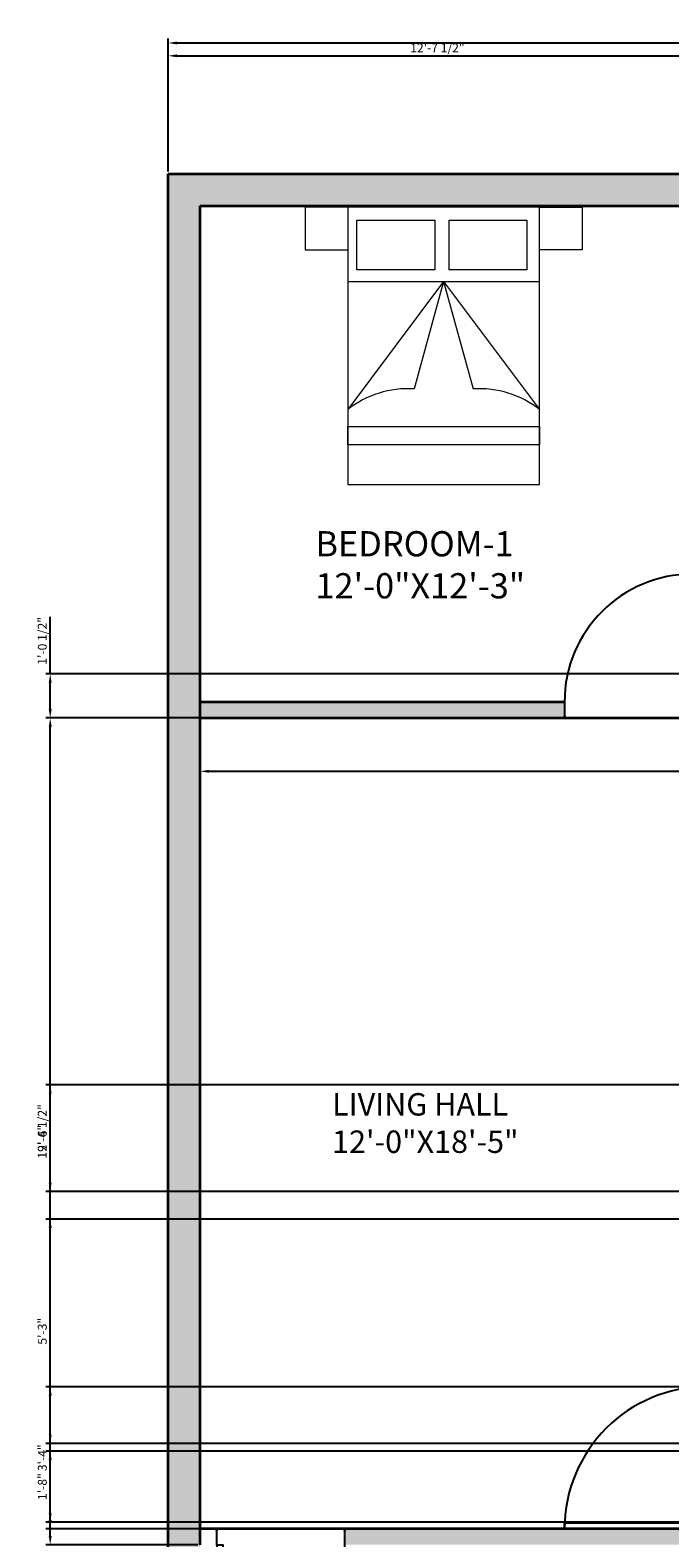
# Model space of a CAD drawing. Units: inches. Extents: x 2063 to 2524, y 2436 to 3097.
# Tile 2 of 4: x 2063 to 2243, y 2673 to 3097. Entities that reach past the tile are written whole.
import ezdxf

# ---------------------------------------------------------------- set-up
doc = ezdxf.new("R2010")
doc.units = ezdxf.units.IN
for name, color, linetype, lineweight in [('A-ANNO-DIMS', 2, 'Continuous', 18), ('A-AREA-IDEN', 7, 'Continuous', 18), ('A-DOOR', 4, 'Continuous', 25), ('A-FURN', 8, 'Continuous', 18), ('A-WALL', 7, 'Continuous', 35)]:
    doc.layers.add(name, color=color, linetype=linetype, lineweight=lineweight)
doc.layers.add('A-WALL-PATT', color=251, linetype='Continuous', lineweight=13, true_color=0x636466)
doc.styles.get("Standard").update_dxf_attribs({"font": 'arial.ttf'})
doc.dimstyles.new('ISO-25', dxfattribs={"dimtxt": 2.5, "dimasz": 2.5, "dimexe": 1.25, "dimexo": 0.625, "dimtad": 1, "dimlunit": 3, "dimtxsty": 'Standard', "dimcen": 2.5, "dimadec": 0, "dimazin": 0, "dimtfac": 1, "dimtmove": 0, "dimatfit": 3, "dimfxl": 1, "dimarcsym": 0})

# ---------------------------------------------------------------- blocks, each defined once
blk = doc.blocks.new('*U3')
for p, q in [((0, 0), (0, -4)), ((-36, 0), (-36, -4))]:
    blk.add_line(p, q)
blk.add_lwpolyline([(0, 0), (0, 36), (-1.75, 36), (-1.75, 0)], close=True)
blk.add_arc((0, 0), 36, 90, 180)
blk = doc.blocks.new('*U5')
for p, q in [((0, 0), (0, -4)), ((40, 0), (40, -4))]:
    blk.add_line(p, q)
blk.add_lwpolyline([(0, 0), (0, 40), (1.75, 40), (1.75, 0)], close=True)
blk.add_arc((0, 0), 40, 0, 90)
blk = doc.blocks.new('*U7')
for p, q in [((0, 0), (0, 4)), ((36, 0), (36, 4))]:
    blk.add_line(p, q)
blk.add_lwpolyline([(0, 0), (0, -36), (1.75, -36), (1.75, 0)], close=True)
blk.add_arc((0, 0), 36, 270, 0)
blk = doc.blocks.new('*D11')
at = {"layer": 'A-ANNO-DIMS', "color": 0, "lineweight": -2, "transparency": 16777216}
for p, q in [((2110.76, 2902.49), (2110.76, 2886.87)), ((2411.76, 2902.49), (2411.76, 2886.87)), ((2113.26, 2888.12), (2409.26, 2888.12))]:
    blk.add_line(p, q, dxfattribs=at)
at = {"layer": 'A-ANNO-DIMS', "color": 0, "transparency": 16777216}
for points in [[(2113.26, 2888.53), (2113.26, 2887.7), (2110.76, 2888.12)], [(2409.26, 2888.53), (2409.26, 2887.7), (2411.76, 2888.12)]]:
    blk.add_solid(points, dxfattribs=at)
at = {"layer": 'Defpoints', "color": 0, "transparency": 16777216}
for p in [(2110.76, 2903.12), (2411.76, 2903.12), (2411.76, 2888.12)]:
    blk.add_point(p, dxfattribs=at)
at = {"layer": 'A-ANNO-DIMS', "color": 0, "transparency": 16777216, "insert": (2261.26, 2890.02), "char_height": 2.5, "attachment_point": 5}
blk.add_mtext('25\'-1"', dxfattribs=at)
blk = doc.blocks.new('*D14')
at = {"layer": 'A-ANNO-DIMS', "color": 0, "lineweight": -2, "transparency": 16777216}
for p, q in [((2101.76, 3056.74), (2101.76, 3094.17)), ((2104.26, 3092.92), (2459.26, 3092.92)), ((2461.76, 3056.74), (2461.76, 3094.17))]:
    blk.add_line(p, q, dxfattribs=at)
at = {"layer": 'A-ANNO-DIMS', "color": 0, "transparency": 16777216}
for points in [[(2104.26, 3093.34), (2104.26, 3092.5), (2101.76, 3092.92)], [(2459.26, 3093.34), (2459.26, 3092.5), (2461.76, 3092.92)]]:
    blk.add_solid(points, dxfattribs=at)
at = {"layer": 'Defpoints', "color": 0, "transparency": 16777216}
for p in [(2461.76, 3092.92), (2101.76, 3056.12), (2461.76, 3056.12)]:
    blk.add_point(p, dxfattribs=at)
at = {"layer": 'A-ANNO-DIMS', "color": 0, "transparency": 16777216, "insert": (2281.76, 3094.82), "char_height": 2.5, "attachment_point": 5}
blk.add_mtext("30'", dxfattribs=at)
blk = doc.blocks.new('BED-DOUBLE-WITH-NIGHTSTANDS')
for p, q in [((12, 78), (0, 78)), ((0, 78), (0, 66)), ((66, 78), (78, 78)), ((78, 78), (78, 66)), ((36.48, 74.39), (36.48, 60.42)), ((40.48, 74.39), (40.48, 60.42)), ((0, 66), (12, 66)), ((77, 66), (66, 66)), ((78, 66), (77, 66)), ((12, 57.08), (66, 57.08)), ((39, 57.08), (12, 21.08)), ((39, 57.08), (30.7, 26.92)), ((39, 57.08), (66, 21.08)), ((39, 57.08), (47.3, 26.92))]:
    blk.add_line(p, q)
for points in [[(12, 0), (66, 0), (66, 78), (12, 78)], [(12, 16.31), (66, 16.31), (66, 11.16), (12, 11.16)]]:
    blk.add_lwpolyline(points, close=True)
for points in [[(36.48, 60.42), (14.53, 60.42), (14.53, 74.39), (36.48, 74.39)], [(40.48, 74.39), (62.43, 74.39), (62.43, 60.42), (40.48, 60.42)]]:
    blk.add_lwpolyline(points)
for centre, start, end in [((29, -0.5), 86.4578, 128.2353), ((49, -0.5), 51.7647, 93.5422)]:
    blk.add_arc(centre, 27.47, start, end)
blk = doc.blocks.new('*D31')
at = {"layer": 'A-ANNO-DIMS', "color": 0, "lineweight": -2, "transparency": 16777216}
for p, q in [((2110.14, 2903.12), (2067.31, 2903.12)), ((2068.56, 2673.12), (2068.56, 2900.62)), ((2110.14, 2670.62), (2067.31, 2670.62))]:
    blk.add_line(p, q, dxfattribs=at)
at = {"layer": 'A-ANNO-DIMS', "color": 0, "transparency": 16777216}
for points in [[(2068.15, 2900.62), (2068.98, 2900.62), (2068.56, 2903.12)], [(2068.15, 2673.12), (2068.98, 2673.12), (2068.56, 2670.62)]]:
    blk.add_solid(points, dxfattribs=at)
at = {"layer": 'Defpoints', "color": 0, "transparency": 16777216}
for p in [(2068.56, 2903.12), (2110.76, 2903.12), (2110.76, 2670.62)]:
    blk.add_point(p, dxfattribs=at)
at = {"layer": 'A-ANNO-DIMS', "color": 0, "transparency": 16777216, "insert": (2066.65, 2786.87), "char_height": 2.5, "attachment_point": 5, "rotation": 90}
blk.add_mtext('19\'-4 1/2"', dxfattribs=at)
blk = doc.blocks.new('*D32')
at = {"layer": 'A-ANNO-DIMS', "color": 0, "lineweight": -2, "transparency": 16777216}
for p, q in [((2101.76, 3056.74), (2101.76, 3090.57)), ((2253.26, 3047.74), (2253.26, 3090.57)), ((2104.26, 3089.32), (2250.76, 3089.32))]:
    blk.add_line(p, q, dxfattribs=at)
at = {"layer": 'A-ANNO-DIMS', "color": 0, "transparency": 16777216}
for points in [[(2104.26, 3089.73), (2104.26, 3088.9), (2101.76, 3089.32)], [(2250.76, 3089.73), (2250.76, 3088.9), (2253.26, 3089.32)]]:
    blk.add_solid(points, dxfattribs=at)
at = {"layer": 'Defpoints', "color": 0, "transparency": 16777216}
for p in [(2253.26, 3089.32), (2101.76, 3056.12), (2253.26, 3047.12)]:
    blk.add_point(p, dxfattribs=at)
at = {"layer": 'A-ANNO-DIMS', "color": 0, "transparency": 16777216, "insert": (2177.51, 3091.24), "char_height": 2.5, "attachment_point": 5}
blk.add_mtext('12\'-7 1/2"', dxfattribs=at)
blk = doc.blocks.new('*D35')
at = {"layer": 'A-ANNO-DIMS', "color": 0, "lineweight": -2, "transparency": 16777216}
for p, q in [((2068.56, 2915.57), (2068.56, 2931.55)), ((2257.14, 2915.57), (2067.31, 2915.57)), ((2068.56, 2905.62), (2068.56, 2913.07)), ((2257.14, 2903.12), (2067.31, 2903.12))]:
    blk.add_line(p, q, dxfattribs=at)
at = {"layer": 'A-ANNO-DIMS', "color": 0, "transparency": 16777216}
for points in [[(2068.15, 2913.07), (2068.98, 2913.07), (2068.56, 2915.57)], [(2068.15, 2905.62), (2068.98, 2905.62), (2068.56, 2903.12)]]:
    blk.add_solid(points, dxfattribs=at)
at = {"layer": 'Defpoints', "color": 0, "transparency": 16777216}
for p in [(2068.56, 2915.57), (2257.76, 2915.57), (2257.76, 2903.12)]:
    blk.add_point(p, dxfattribs=at)
at = {"layer": 'A-ANNO-DIMS', "color": 0, "transparency": 16777216, "insert": (2066.65, 2924.81), "char_height": 2.5, "attachment_point": 5, "rotation": 90}
blk.add_mtext('1\'-0 1/2"', dxfattribs=at)
blk = doc.blocks.new('*D41')
at = {"layer": 'A-ANNO-DIMS', "color": 0, "lineweight": -2, "transparency": 16777216}
for p, q in [((2305.15, 2799.95), (2067.31, 2799.95)), ((2068.56, 2772.45), (2068.56, 2797.45)), ((2305.14, 2769.95), (2067.31, 2769.95))]:
    blk.add_line(p, q, dxfattribs=at)
at = {"layer": 'A-ANNO-DIMS', "color": 0, "transparency": 16777216}
for points in [[(2068.15, 2797.45), (2068.98, 2797.45), (2068.56, 2799.95)], [(2068.15, 2772.45), (2068.98, 2772.45), (2068.56, 2769.95)]]:
    blk.add_solid(points, dxfattribs=at)
at = {"layer": 'Defpoints', "color": 0, "transparency": 16777216}
for p in [(2068.56, 2799.95), (2305.78, 2799.95), (2305.76, 2769.95)]:
    blk.add_point(p, dxfattribs=at)
at = {"layer": 'A-ANNO-DIMS', "color": 0, "transparency": 16777216, "insert": (2066.66, 2784.95), "char_height": 2.5, "attachment_point": 5, "rotation": 90}
blk.add_mtext('2\'-6"', dxfattribs=at)
blk = doc.blocks.new('*D42')
at = {"layer": 'A-ANNO-DIMS', "color": 0, "lineweight": -2, "transparency": 16777216}
for p, q in [((2426.27, 2762.21), (2067.31, 2762.21)), ((2068.56, 2701.62), (2068.56, 2759.71)), ((2426.27, 2699.12), (2067.31, 2699.12))]:
    blk.add_line(p, q, dxfattribs=at)
at = {"layer": 'A-ANNO-DIMS', "color": 0, "transparency": 16777216}
for points in [[(2068.15, 2759.71), (2068.98, 2759.71), (2068.56, 2762.21)], [(2068.15, 2701.62), (2068.98, 2701.62), (2068.56, 2699.12)]]:
    blk.add_solid(points, dxfattribs=at)
at = {"layer": 'Defpoints', "color": 0, "transparency": 16777216}
for p in [(2068.56, 2762.21), (2426.9, 2762.21), (2426.9, 2699.12)]:
    blk.add_point(p, dxfattribs=at)
at = {"layer": 'A-ANNO-DIMS', "color": 0, "transparency": 16777216, "insert": (2066.66, 2730.67), "char_height": 2.5, "attachment_point": 5, "rotation": 90}
blk.add_mtext('5\'-3"', dxfattribs=at)
blk = doc.blocks.new('*D45')
at = {"layer": 'A-ANNO-DIMS', "color": 0, "lineweight": -2, "transparency": 16777216}
for p, q in [((2252.63, 2715.09), (2067.31, 2715.09)), ((2068.56, 2677.62), (2068.56, 2712.59)), ((2252.64, 2675.12), (2067.31, 2675.12))]:
    blk.add_line(p, q, dxfattribs=at)
at = {"layer": 'A-ANNO-DIMS', "color": 0, "transparency": 16777216}
for points in [[(2068.15, 2712.59), (2068.98, 2712.59), (2068.56, 2715.09)], [(2068.15, 2677.62), (2068.98, 2677.62), (2068.56, 2675.12)]]:
    blk.add_solid(points, dxfattribs=at)
at = {"layer": 'Defpoints', "color": 0, "transparency": 16777216}
for p in [(2068.56, 2715.09), (2253.26, 2715.09), (2253.26, 2675.12)]:
    blk.add_point(p, dxfattribs=at)
at = {"layer": 'A-ANNO-DIMS', "color": 0, "transparency": 16777216, "insert": (2066.66, 2695.1), "char_height": 2.5, "attachment_point": 5, "rotation": 90}
blk.add_mtext('3\'-4"', dxfattribs=at)
blk = doc.blocks.new('*D50')
at = {"layer": 'A-ANNO-DIMS', "color": 0, "lineweight": -2, "transparency": 16777216}
for p, q in [((2334.17, 2696.99), (2067.31, 2696.99)), ((2068.56, 2679.49), (2068.56, 2694.49)), ((2334.17, 2676.99), (2067.31, 2676.99))]:
    blk.add_line(p, q, dxfattribs=at)
at = {"layer": 'A-ANNO-DIMS', "color": 0, "transparency": 16777216}
for points in [[(2068.15, 2694.49), (2068.98, 2694.49), (2068.56, 2696.99)], [(2068.15, 2679.49), (2068.98, 2679.49), (2068.56, 2676.99)]]:
    blk.add_solid(points, dxfattribs=at)
at = {"layer": 'Defpoints', "color": 0, "transparency": 16777216}
for p in [(2068.56, 2696.99), (2334.8, 2696.99), (2334.8, 2676.99)]:
    blk.add_point(p, dxfattribs=at)
at = {"layer": 'A-ANNO-DIMS', "color": 0, "transparency": 16777216, "insert": (2066.66, 2686.99), "char_height": 2.5, "attachment_point": 5, "rotation": 90}
blk.add_mtext('1\'-8"', dxfattribs=at)

msp = doc.modelspace()

# ---------------------------------------------------------------- hatches: boundary and pattern name
at = {"layer": 'A-WALL-PATT'}
h = msp.add_hatch(color=256, dxfattribs=at)
h.dxf.hatch_style = 1
h.paths.add_polyline_path([(2110.763, 2670.618), (2110.763, 2676.643), (2110.763, 3047.118), (2452.763, 3047.118), (2452.763, 2501.118), (2200.478, 2501.118), (2200.478, 2492.118), (2461.763, 2492.118), (2461.763, 3056.118), (2101.763, 3056.118), (2101.763, 2492.118), (2149.478, 2492.118), (2149.478, 2496.618), (2149.478, 2501.118), (2110.763, 2501.118)])
h.paths.add_polyline_path([(2257.763, 2675.118), (2257.255, 2675.091), (2253.255, 2675.091), (2213.255, 2675.091), (2151.474, 2675.107), (2151.474, 2674.543), (2151.474, 2670.618), (2253.263, 2670.618), (2253.263, 2501.118), (2257.763, 2501.118)], flags=17)
h.paths.add_polyline_path([(2310.263, 3006.972), (2305.763, 3006.972), (2305.763, 2920.067), (2301.763, 2920.067), (2301.759, 2920.067), (2301.759, 2920.063), (2301.759, 2916.063), (2301.759, 2915.567), (2305.763, 2915.567), (2305.763, 2903.118), (2314.3, 2903.118), (2314.3, 2903.618), (2314.3, 2907.618), (2310.263, 2907.618)], flags=17)
h.paths.add_polyline_path([(2257.763, 3006.972), (2253.263, 3006.972), (2253.263, 2907.618), (2249.263, 2907.618), (2249.258, 2907.618), (2249.258, 2907.597), (2249.258, 2903.597), (2249.258, 2903.118), (2257.763, 2903.118), (2257.763, 2915.567), (2271.759, 2915.567), (2271.759, 2916.063), (2271.759, 2920.067), (2257.763, 2920.067)], flags=17)
h.paths.add_polyline_path([(2213.258, 2907.618), (2110.763, 2907.618), (2110.763, 2903.118), (2213.258, 2903.118), (2213.258, 2903.597)], flags=17)
h.paths.add_polyline_path([(2411.763, 2907.618), (2350.3, 2907.618), (2350.3, 2903.618), (2350.3, 2903.118), (2407.264, 2903.118), (2411.763, 2903.118)], flags=17)
h.paths.add_polyline_path([(2260.327, 2964.034), (2307.905, 2964.034), (2307.905, 2989.359), (2260.327, 2989.359)], flags=25)

# ---------------------------------------------------------------- linework, layer by layer
at = {"layer": 'A-WALL'}
for p, q in [((2101.763, 3056.118), (2461.763, 3056.118)), ((2101.763, 2492.118), (2101.763, 3056.118)), ((2110.763, 3047.118), (2452.763, 3047.118)), ((2110.763, 2675.118), (2110.763, 3047.118)), ((2110.763, 2907.618), (2213.258, 2907.618)), ((2110.763, 2903.118), (2257.763, 2903.118)), ((2213.258, 2903.597), (2213.258, 2903.118)), ((2110.763, 2670.618), (2110.763, 2676.643)), ((2257.763, 2675.118), (2110.763, 2675.118)), ((2115.474, 2674.543), (2115.474, 2675.118)), ((2151.474, 2674.543), (2151.474, 2675.118))]:
    msp.add_line(p, q, dxfattribs=at)

# ---------------------------------------------------------------- block references
at = {"layer": 'A-DOOR'}
for name, p in [('*U3', (2249.258, 2907.597)), ('*U7', (2115.474, 2670.543))]:
    msp.add_blockref(name, p, dxfattribs=at)
at = {"layer": 'A-DOOR', "rotation": 90}
msp.add_blockref('*U5', (2253.255, 2675.091), dxfattribs=at)
at = {"layer": 'A-FURN'}
msp.add_blockref('BED-DOUBLE-WITH-NIGHTSTANDS', (2140.256, 2968.743), dxfattribs=at)

# ---------------------------------------------------------------- texts
at = {"layer": 'A-AREA-IDEN', "insert": (2143.177, 2955.649), "char_height": 7.08715, "attachment_point": 1}
msp.add_mtext('BEDROOM-1\\P12\'-0"X12\'-3"', dxfattribs=at)
at = {"layer": 'A-AREA-IDEN', "insert": (2147.871, 2797.625), "char_height": 6.30204, "attachment_point": 1}
msp.add_mtext_dynamic_manual_height_columns('LIVING HALL\\P12\'-0"X18\'-5"', width=63.96398, gutter_width=31.51, heights=[0], dxfattribs=at)

# ---------------------------------------------------------------- dimensions: what is measured, and where the dimension line sits
at = {"layer": 'A-ANNO-DIMS'}
for base, p1, p2, override, picture, middle in [((2461.763, 3092.92), (2101.763, 3056.118), (2461.763, 3056.118), {"dimclrd": 0, "dimclre": 0, "dimclrt": 0}, '*D14', (2281.763, 3094.823)), ((2253.263, 3089.318), (2101.763, 3056.118), (2253.263, 3047.118), {"dimdec": 1, "dimlfac": 1, "dimrnd": 0, "dimzin": 1, "dimdsep": 46, "dimlunit": 4, "dimfrac": 2}, '*D32', (2177.513, 3091.235)), ((2411.763, 2888.116), (2110.763, 2903.118), (2411.763, 2903.118), {"dimclrd": 0, "dimclre": 0, "dimclrt": 0}, '*D11', (2261.263, 2890.017))]:
    dim = msp.add_linear_dim(base=base, p1=p1, p2=p2, dimstyle='ISO-25', override=override, dxfattribs=at)
    dim.commit()
    dim.dimension.update_dxf_attribs({"geometry": picture, "text_midpoint": middle})
for base, p1, p2, picture, middle in [((2068.563, 2915.567), (2257.763, 2903.118), (2257.763, 2915.567), '*D35', (2066.646, 2924.81)), ((2068.563, 2903.118), (2110.763, 2670.618), (2110.763, 2903.118), '*D31', (2066.646, 2786.868)), ((2068.563, 2799.95), (2305.763, 2769.95), (2305.776, 2799.95), '*D41', (2066.662, 2784.95)), ((2068.563, 2762.214), (2426.899, 2699.118), (2426.899, 2762.214), '*D42', (2066.661, 2730.666)), ((2068.563, 2715.091), (2253.263, 2675.118), (2253.255, 2715.091), '*D45', (2066.661, 2695.104)), ((2068.563, 2696.991), (2334.798, 2676.988), (2334.798, 2696.991), '*D50', (2066.662, 2686.99))]:
    dim = msp.add_linear_dim(base=base, p1=p1, p2=p2, angle=90, dimstyle='ISO-25', override={"dimdec": 1, "dimlfac": 1, "dimrnd": 0, "dimzin": 1, "dimdsep": 46, "dimlunit": 4, "dimfrac": 2}, dxfattribs=at)
    dim.commit()
    dim.dimension.update_dxf_attribs({"geometry": picture, "text_midpoint": middle})

doc.saveas('drawing.dxf')
